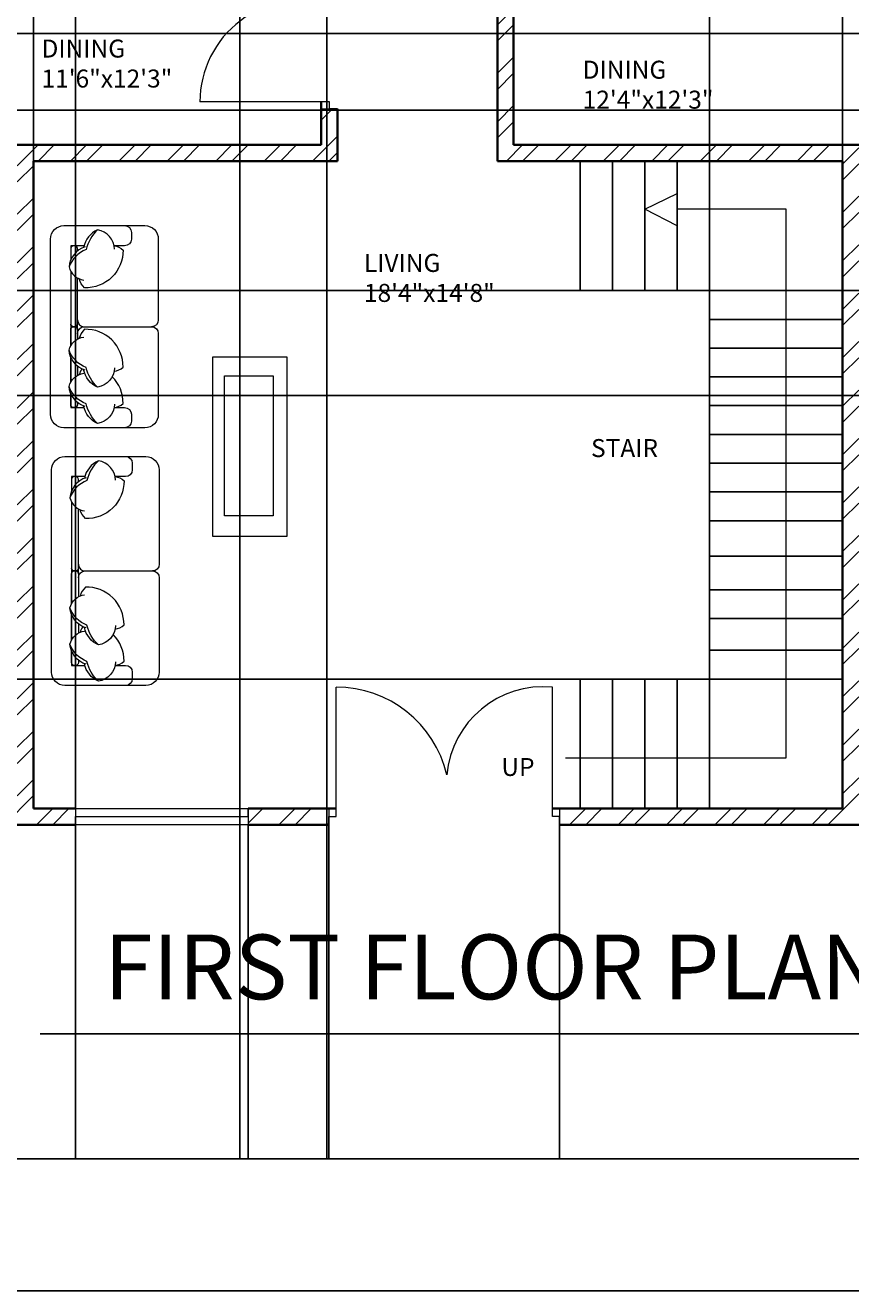
# Model space of a CAD drawing. Units: inches. Extents: x 1965 to 2673, y 1802 to 2669.
# Tile 4 of 16: x 2198 to 2427, y 1802 to 2154. Entities that reach past the tile are written whole.
import ezdxf

# ---------------------------------------------------------------- set-up
doc = ezdxf.new("R2010")
doc.units = ezdxf.units.IN
for name, color, linetype, lineweight in [('A-ANNO-DIMS', 2, 'Continuous', 18), ('A-ANNO-SYMB', 7, 'Continuous', 18), ('A-ANNO-TTLB', 7, 'Continuous', 25), ('A-AREA-IDEN', 7, 'Continuous', 18), ('A-DOOR', 11, 'Continuous', 18), ('A-FLOR-STRS', 131, 'Continuous', 25), ('A-FURN', 8, 'Continuous', 13), ('A-GLAZ', 181, 'Continuous', 18), ('A-WALL', 7, 'Continuous', 35), ('A-WALL-PATT', 252, 'Continuous', 13)]:
    doc.layers.add(name, color=color, linetype=linetype, lineweight=lineweight)
doc.styles.get("Standard").update_dxf_attribs({"font": 'arial.ttf'})
doc.dimstyles.get("Standard").update_dxf_attribs({"dimtxt": 0.18, "dimasz": 0.18, "dimexe": 0.18, "dimexo": 0.0625, "dimgap": 0.09, "dimtad": 0, "dimtih": 1, "dimtoh": 1, "dimdec": 4, "dimzin": 0, "dimdsep": 46, "dimtxsty": 'Standard', "dimcen": 0.09, "dimadec": 0, "dimazin": 0, "dimtfac": 1, "dimtdec": 4, "dimtofl": 0, "dimtmove": 0, "dimatfit": 3, "dimfxl": 1, "dimtolj": 1, "dimtzin": 0, "dimarcsym": 0})

# ---------------------------------------------------------------- blocks, each defined once
blk = doc.blocks.new('*D25')
at = {"layer": 'A-ANNO-DIMS', "color": 0, "lineweight": -2, "transparency": 16777216}
for p, q in [((2047.09, 1931.53), (2047.09, 1838.49)), ((2578.09, 1931.53), (2578.09, 1838.49)), ((2047.27, 1838.67), (2312.32, 1838.67)), ((2577.91, 1838.67), (2312.86, 1838.67))]:
    blk.add_line(p, q, dxfattribs=at)
at = {"layer": 'A-ANNO-DIMS', "color": 0, "transparency": 16777216}
for points in [[(2047.27, 1838.7), (2047.27, 1838.64), (2047.09, 1838.67)], [(2577.91, 1838.7), (2577.91, 1838.64), (2578.09, 1838.67)]]:
    blk.add_solid(points, dxfattribs=at)
at = {"layer": 'Defpoints', "color": 0, "transparency": 16777216}
for p in [(2047.09, 1931.59), (2578.09, 1931.59), (2578.09, 1838.67)]:
    blk.add_point(p, dxfattribs=at)
at = {"layer": 'A-ANNO-DIMS', "color": 0, "transparency": 16777216, "insert": (2312.59, 1838.67), "char_height": 0.18, "attachment_point": 5}
blk.add_mtext('\\A1;531', dxfattribs=at)
blk = doc.blocks.new('*D40')
at = {"layer": 'A-ANNO-DIMS', "color": 0, "lineweight": -2, "transparency": 16777216}
for p, q in [((2200.09, 1936.15), (2200.09, 2600.5)), ((2200.27, 2600.32), (2205.48, 2600.32)), ((2211.59, 2600.32), (2206.38, 2600.32)), ((2211.77, 1936.15), (2211.77, 2600.5))]:
    blk.add_line(p, q, dxfattribs=at)
at = {"layer": 'A-ANNO-DIMS', "color": 0, "transparency": 16777216}
for points in [[(2200.27, 2600.35), (2200.27, 2600.29), (2200.09, 2600.32)], [(2211.59, 2600.35), (2211.59, 2600.29), (2211.77, 2600.32)]]:
    blk.add_solid(points, dxfattribs=at)
at = {"layer": 'Defpoints', "color": 0, "transparency": 16777216}
for p in [(2211.77, 2600.32), (2200.09, 1936.09), (2211.77, 1936.09)]:
    blk.add_point(p, dxfattribs=at)
at = {"layer": 'A-ANNO-DIMS', "color": 0, "transparency": 16777216, "insert": (2205.93, 2600.32), "char_height": 0.18, "attachment_point": 5}
blk.add_mtext('\\A1;11.674', dxfattribs=at)
blk = doc.blocks.new('*D41')
at = {"layer": 'A-ANNO-DIMS', "color": 0, "lineweight": -2, "transparency": 16777216}
for p, q in [((2211.77, 1931.53), (2211.77, 1838.49)), ((2259.77, 1931.53), (2259.77, 1838.49)), ((2211.95, 1838.67), (2235.54, 1838.67)), ((2259.59, 1838.67), (2235.99, 1838.67))]:
    blk.add_line(p, q, dxfattribs=at)
at = {"layer": 'A-ANNO-DIMS', "color": 0, "transparency": 16777216}
for points in [[(2211.95, 1838.7), (2211.95, 1838.64), (2211.77, 1838.67)], [(2259.59, 1838.7), (2259.59, 1838.64), (2259.77, 1838.67)]]:
    blk.add_solid(points, dxfattribs=at)
at = {"layer": 'Defpoints', "color": 0, "transparency": 16777216}
for p in [(2211.77, 1931.59), (2259.77, 1931.59), (2259.77, 1838.67)]:
    blk.add_point(p, dxfattribs=at)
at = {"layer": 'A-ANNO-DIMS', "color": 0, "transparency": 16777216, "insert": (2235.77, 1838.67), "char_height": 0.18, "attachment_point": 5}
blk.add_mtext('\\A1;48', dxfattribs=at)
blk = doc.blocks.new('*D42')
at = {"layer": 'A-ANNO-DIMS', "color": 0, "lineweight": -2, "transparency": 16777216}
for p, q in [((2259.77, 1931.53), (2259.77, 1838.49)), ((2282.25, 1931.53), (2282.25, 1838.49)), ((2259.95, 1838.67), (2270.54, 1838.67)), ((2282.07, 1838.67), (2271.47, 1838.67))]:
    blk.add_line(p, q, dxfattribs=at)
at = {"layer": 'A-ANNO-DIMS', "color": 0, "transparency": 16777216}
for points in [[(2259.95, 1838.7), (2259.95, 1838.64), (2259.77, 1838.67)], [(2282.07, 1838.7), (2282.07, 1838.64), (2282.25, 1838.67)]]:
    blk.add_solid(points, dxfattribs=at)
at = {"layer": 'Defpoints', "color": 0, "transparency": 16777216}
for p in [(2259.77, 1931.59), (2282.25, 1931.59), (2282.25, 1838.67)]:
    blk.add_point(p, dxfattribs=at)
at = {"layer": 'A-ANNO-DIMS', "color": 0, "transparency": 16777216, "insert": (2271.01, 1838.67), "char_height": 0.18, "attachment_point": 5}
blk.add_mtext('\\A1;22.483', dxfattribs=at)
blk = doc.blocks.new('*D43')
at = {"layer": 'A-ANNO-DIMS', "color": 0, "lineweight": -2, "transparency": 16777216}
for p, q in [((2282.25, 1931.53), (2282.25, 1838.49)), ((2346.41, 1931.53), (2346.41, 1838.49)), ((2282.43, 1838.67), (2313.93, 1838.67)), ((2346.23, 1838.67), (2314.72, 1838.67))]:
    blk.add_line(p, q, dxfattribs=at)
at = {"layer": 'A-ANNO-DIMS', "color": 0, "transparency": 16777216}
for points in [[(2282.43, 1838.7), (2282.43, 1838.64), (2282.25, 1838.67)], [(2346.23, 1838.7), (2346.23, 1838.64), (2346.41, 1838.67)]]:
    blk.add_solid(points, dxfattribs=at)
at = {"layer": 'Defpoints', "color": 0, "transparency": 16777216}
for p in [(2282.25, 1931.59), (2346.41, 1931.59), (2346.41, 1838.67)]:
    blk.add_point(p, dxfattribs=at)
at = {"layer": 'A-ANNO-DIMS', "color": 0, "transparency": 16777216, "insert": (2314.33, 1838.67), "char_height": 0.18, "attachment_point": 5}
blk.add_mtext('\\A1;64.16', dxfattribs=at)
blk = doc.blocks.new('*D45')
at = {"layer": 'A-ANNO-DIMS', "color": 0, "lineweight": -2, "transparency": 16777216}
for p, q in [((2573.53, 2080.09), (2012.19, 2080.09)), ((2012.37, 2079.91), (2012.37, 2065.68)), ((2012.37, 2051.08), (2012.37, 2065.31)), ((2573.53, 2050.9), (2012.19, 2050.9))]:
    blk.add_line(p, q, dxfattribs=at)
at = {"layer": 'A-ANNO-DIMS', "color": 0, "transparency": 16777216}
for points in [[(2012.34, 2079.91), (2012.4, 2079.91), (2012.37, 2080.09)], [(2012.34, 2051.08), (2012.4, 2051.08), (2012.37, 2050.9)]]:
    blk.add_solid(points, dxfattribs=at)
at = {"layer": 'Defpoints', "color": 0, "transparency": 16777216}
for p in [(2012.37, 2080.09), (2573.59, 2080.09), (2573.59, 2050.9)]:
    blk.add_point(p, dxfattribs=at)
at = {"layer": 'A-ANNO-DIMS', "color": 0, "transparency": 16777216, "insert": (2012.37, 2065.49), "char_height": 0.18, "attachment_point": 5}
blk.add_mtext('\\A1;29.19', dxfattribs=at)
blk = doc.blocks.new('*D46')
at = {"layer": 'A-ANNO-DIMS', "color": 0, "lineweight": -2, "transparency": 16777216}
for p, q in [((2573.53, 2151.59), (2012.19, 2151.59)), ((2012.37, 2151.41), (2012.37, 2141.12)), ((2012.37, 2130.47), (2012.37, 2140.76)), ((2573.53, 2130.29), (2012.19, 2130.29))]:
    blk.add_line(p, q, dxfattribs=at)
at = {"layer": 'A-ANNO-DIMS', "color": 0, "transparency": 16777216}
for points in [[(2012.34, 2151.41), (2012.4, 2151.41), (2012.37, 2151.59)], [(2012.34, 2130.47), (2012.4, 2130.47), (2012.37, 2130.29)]]:
    blk.add_solid(points, dxfattribs=at)
at = {"layer": 'Defpoints', "color": 0, "transparency": 16777216}
for p in [(2012.37, 2151.59), (2573.59, 2151.59), (2573.59, 2130.29)]:
    blk.add_point(p, dxfattribs=at)
at = {"layer": 'A-ANNO-DIMS', "color": 0, "transparency": 16777216, "insert": (2012.37, 2140.94), "char_height": 0.18, "attachment_point": 5}
blk.add_mtext('\\A1;21.3', dxfattribs=at)
blk = doc.blocks.new('*D50')
at = {"layer": 'A-ANNO-DIMS', "color": 0, "lineweight": -2, "transparency": 16777216}
for p, q in [((2388.09, 2116.15), (2388.09, 2600.5)), ((2388.27, 2600.32), (2406.37, 2600.32)), ((2424.91, 2600.32), (2406.81, 2600.32)), ((2425.09, 2116.15), (2425.09, 2600.5))]:
    blk.add_line(p, q, dxfattribs=at)
at = {"layer": 'A-ANNO-DIMS', "color": 0, "transparency": 16777216}
for points in [[(2388.27, 2600.35), (2388.27, 2600.29), (2388.09, 2600.32)], [(2424.91, 2600.35), (2424.91, 2600.29), (2425.09, 2600.32)]]:
    blk.add_solid(points, dxfattribs=at)
at = {"layer": 'Defpoints', "color": 0, "transparency": 16777216}
for p in [(2425.09, 2600.32), (2388.09, 2116.09), (2425.09, 2116.09)]:
    blk.add_point(p, dxfattribs=at)
at = {"layer": 'A-ANNO-DIMS', "color": 0, "transparency": 16777216, "insert": (2406.59, 2600.32), "char_height": 0.18, "attachment_point": 5}
blk.add_mtext('\\A1;37', dxfattribs=at)
blk = doc.blocks.new('*D51')
at = {"layer": 'A-ANNO-DIMS', "color": 0, "lineweight": -2, "transparency": 16777216}
for p, q in [((2388.03, 2080.09), (2012.19, 2080.09)), ((2012.37, 2079.91), (2012.37, 2026.27)), ((2012.37, 1972.27), (2012.37, 2025.91)), ((2388.03, 1972.09), (2012.19, 1972.09))]:
    blk.add_line(p, q, dxfattribs=at)
at = {"layer": 'A-ANNO-DIMS', "color": 0, "transparency": 16777216}
for points in [[(2012.34, 2079.91), (2012.4, 2079.91), (2012.37, 2080.09)], [(2012.34, 1972.27), (2012.4, 1972.27), (2012.37, 1972.09)]]:
    blk.add_solid(points, dxfattribs=at)
at = {"layer": 'Defpoints', "color": 0, "transparency": 16777216}
for p in [(2012.37, 2080.09), (2388.09, 2080.09), (2388.09, 1972.09)]:
    blk.add_point(p, dxfattribs=at)
at = {"layer": 'A-ANNO-DIMS', "color": 0, "transparency": 16777216, "insert": (2012.37, 2026.09), "char_height": 0.18, "attachment_point": 5}
blk.add_mtext('\\A1;108', dxfattribs=at)
blk = doc.blocks.new('*D53')
at = {"layer": 'A-ANNO-DIMS', "color": 0, "lineweight": -2, "transparency": 16777216}
for p, q in [((2257.52, 2457.53), (2257.52, 1838.49)), ((2281.66, 2457.53), (2281.66, 1838.49)), ((2257.7, 1838.67), (2269.12, 1838.67)), ((2281.48, 1838.67), (2270.05, 1838.67))]:
    blk.add_line(p, q, dxfattribs=at)
at = {"layer": 'A-ANNO-DIMS', "color": 0, "transparency": 16777216}
for points in [[(2257.7, 1838.7), (2257.7, 1838.64), (2257.52, 1838.67)], [(2281.48, 1838.7), (2281.48, 1838.64), (2281.66, 1838.67)]]:
    blk.add_solid(points, dxfattribs=at)
at = {"layer": 'Defpoints', "color": 0, "transparency": 16777216}
for p in [(2257.52, 2457.59), (2281.66, 2457.59), (2281.66, 1838.67)]:
    blk.add_point(p, dxfattribs=at)
at = {"layer": 'A-ANNO-DIMS', "color": 0, "transparency": 16777216, "insert": (2269.59, 1838.67), "char_height": 0.18, "attachment_point": 5}
blk.add_mtext('\\A1;24.145', dxfattribs=at)

msp = doc.modelspace()

# ---------------------------------------------------------------- hatches: boundary and pattern name
at = {"layer": 'A-WALL-PATT'}
h = msp.add_hatch(dxfattribs=at)
h.set_pattern_fill('ANSI32', color=256)
h.paths.add_polyline_path([(2051.5927, 2561.0914), (2076.7559, 2561.0914), (2076.7559, 2563.3414), (2076.7559, 2565.5914), (2047.0927, 2565.5914), (2047.0927, 2518.3824), (2051.5927, 2518.3824)])
h.paths.add_polyline_path([(2051.5927, 2458.3824), (2049.3427, 2458.3824), (2047.0927, 2458.3824), (2047.0927, 2412.5914), (2248.0927, 2412.5914), (2248.0927, 2268.5914), (2252.5927, 2268.5914), (2252.5927, 2412.5914), (2252.5927, 2421.0404), (2250.3427, 2421.0404), (2248.0927, 2421.0404), (2248.0927, 2417.0914), (2051.5927, 2417.0914)])
h.paths.add_polyline_path([(2211.4933, 2268.5914), (2104.0927, 2268.5914), (2104.0927, 2272.4654), (2101.8427, 2272.4654), (2099.5927, 2272.4654), (2099.5927, 2268.5914), (2051.5927, 2268.5914), (2051.5927, 2264.0914), (2147.5927, 2264.0914), (2147.5927, 2259.8893), (2152.0927, 2259.8893), (2152.0927, 2264.0914), (2211.4933, 2264.0914), (2211.4933, 2266.3414)])
h.paths.add_polyline_path([(2104.0927, 2376.0914), (2099.5927, 2376.0914), (2047.0927, 2376.0914), (2047.0927, 2333.0682), (2051.5927, 2333.0682), (2051.5927, 2371.5914), (2099.5927, 2371.5914), (2099.5927, 2293.6123), (2104.0927, 2293.6123)], flags=17)
h.paths.add_polyline_path([(2051.5927, 2309.0682), (2047.0927, 2309.0682), (2047.0927, 2233.5821), (2051.5927, 2233.5821)])
h.paths.add_polyline_path([(2104.0927, 2412.5914), (2099.5927, 2412.5914), (2099.5927, 2376.0914), (2104.0927, 2376.0914)], flags=17)
h.paths.add_polyline_path([(2290.1254, 2268.5914), (2242.4924, 2268.5914), (2242.4924, 2264.0914), (2290.1254, 2264.0914), (2290.1254, 2266.3414)])
h.paths.add_polyline_path([(2284.653, 2264.0914), (2280.153, 2264.0914), (2280.153, 2161.6826), (2284.653, 2161.6826)])
h.paths.add_polyline_path([(2578.0927, 2329.4656), (2573.5927, 2329.4656), (2573.5927, 2268.5914), (2525.5927, 2268.5914), (2525.5927, 2271.9222), (2523.3427, 2271.9222), (2521.0927, 2271.9222), (2521.0927, 2268.5914), (2324.2835, 2268.5914), (2324.2835, 2264.0914), (2329.0927, 2264.0914), (2329.0927, 2259.4977), (2333.5927, 2259.4977), (2333.5927, 2264.0914), (2473.0927, 2264.0914), (2473.0927, 2259.9371), (2477.5927, 2259.9371), (2477.5927, 2264.0914), (2573.5927, 2264.0914), (2573.5927, 2235.5751), (2578.0927, 2235.5751)])
h.paths.add_polyline_path([(2377.0927, 2412.5914), (2578.0927, 2412.5914), (2578.0927, 2444.2286), (2575.8427, 2444.2286), (2573.5927, 2444.2286), (2573.5927, 2417.0914), (2429.5927, 2417.0914), (2377.0927, 2417.0914), (2377.0927, 2421.7443), (2372.5927, 2421.7443), (2372.5927, 2268.5914), (2377.0927, 2268.5914)])
h.paths.add_polyline_path([(2525.5927, 2371.5914), (2573.5927, 2371.5914), (2573.5927, 2353.4656), (2578.0927, 2353.4656), (2578.0927, 2376.0914), (2525.5927, 2376.0914), (2521.0927, 2376.0914), (2521.0927, 2290.6472), (2525.5927, 2290.6472)], flags=17)
h.paths.add_polyline_path([(2477.5927, 2236.4106), (2475.3427, 2236.4106), (2473.0927, 2236.4106), (2473.0927, 2084.5914), (2465.3309, 2084.5914), (2465.3309, 2080.0914), (2481.6764, 2080.0914), (2481.6764, 2082.3414), (2481.6764, 2084.5914), (2477.5927, 2084.5914), (2477.5927, 2151.5914), (2573.5927, 2151.5914), (2573.5927, 2130.2907), (2578.0927, 2130.2907), (2578.0927, 2199.5751), (2575.8427, 2199.5751), (2573.5927, 2199.5751), (2573.5927, 2156.0914), (2477.5927, 2156.0914)])
h.paths.add_polyline_path([(2573.5927, 2084.5914), (2505.5513, 2084.5914), (2505.5513, 2080.0914), (2573.5927, 2080.0914)], flags=17)
h.paths.add_polyline_path([(2578.0927, 2106.2907), (2575.8427, 2106.2907), (2573.5927, 2106.2907), (2573.5927, 2050.8986), (2578.0927, 2050.8986)])
h.paths.add_polyline_path([(2578.0927, 1990.8986), (2575.8427, 1990.8986), (2573.5927, 1990.8986), (2573.5927, 1936.0914), (2522.132, 1936.0914), (2522.132, 1931.5914), (2578.0927, 1931.5914)])
h.paths.add_polyline_path([(2462.132, 1936.0914), (2429.5927, 1936.0914), (2429.5927, 2080.0914), (2432.623, 2080.0914), (2432.623, 2082.3414), (2432.623, 2084.5914), (2429.5927, 2084.5914), (2429.5927, 2120.5914), (2333.5927, 2120.5914), (2333.5927, 2229.3125), (2331.3427, 2229.3125), (2329.0927, 2229.3125), (2329.0927, 2116.0914), (2425.0927, 2116.0914), (2425.0927, 1936.0914), (2346.4058, 1936.0914), (2346.4058, 1931.5914), (2462.132, 1931.5914), (2462.132, 1933.8414)])
h.paths.add_polyline_path([(2211.767, 1933.8414), (2211.767, 1936.0914), (2200.0927, 1936.0914), (2200.0927, 2080.0914), (2200.0927, 2116.0914), (2284.653, 2116.0914), (2284.653, 2130.591), (2282.403, 2130.591), (2280.153, 2130.591), (2280.153, 2120.5914), (2200.0927, 2120.5914), (2195.5927, 2120.5914), (2195.5927, 2080.0914), (2195.5927, 1936.0914), (2139.0533, 1936.0914), (2139.0533, 1931.5914), (2211.767, 1931.5914)])
h.paths.add_polyline_path([(2282.2502, 1933.8414), (2282.2502, 1936.0914), (2259.767, 1936.0914), (2259.767, 1931.5914), (2282.2502, 1931.5914)], flags=17)
h.paths.add_polyline_path([(2051.5927, 1987.096), (2049.3427, 1987.096), (2047.0927, 1987.096), (2047.0927, 1931.5914), (2079.0533, 1931.5914), (2079.0533, 1933.8414), (2079.0533, 1936.0914), (2051.5927, 1936.0914)])
h.paths.add_polyline_path([(2051.5927, 2197.5821), (2049.3427, 2197.5821), (2047.0927, 2197.5821), (2047.0927, 2141.952), (2051.5927, 2141.952), (2051.5927, 2151.5914), (2147.5927, 2151.5914), (2147.5927, 2084.5914), (2144.3652, 2084.5914), (2144.3652, 2080.0914), (2155.9662, 2080.0914), (2155.9662, 2082.3414), (2155.9662, 2084.5914), (2152.0927, 2084.5914), (2152.0927, 2239.4921), (2149.8427, 2239.4921), (2147.5927, 2239.4921), (2147.5927, 2156.0914), (2051.5927, 2156.0914)])
h.paths.add_polyline_path([(2051.5927, 2080.0914), (2123.8575, 2080.0914), (2123.8575, 2082.3414), (2123.8575, 2084.5914), (2051.5927, 2084.5914), (2051.5927, 2117.952), (2047.0927, 2117.952), (2047.0927, 2047.096), (2051.5927, 2047.096)])
h = msp.add_hatch(dxfattribs=at)
h.set_pattern_fill('ANSI32', color=256)
h.paths.add_polyline_path([(2210.2316, 2563.3414), (2210.2316, 2565.5914), (2136.7559, 2565.5914), (2136.7559, 2561.0914), (2195.5927, 2561.0914), (2195.5927, 2485.8604), (2200.0927, 2485.8604), (2200.0927, 2561.0914), (2210.2316, 2561.0914)])
h.paths.add_polyline_path([(2285.9734, 2565.5914), (2234.2316, 2565.5914), (2234.2316, 2561.0914), (2248.0927, 2561.0914), (2248.0927, 2462.0914), (2200.0927, 2462.0914), (2200.0927, 2465.2357), (2197.8427, 2465.2357), (2195.5927, 2465.2357), (2195.5927, 2457.5914), (2248.0927, 2457.5914), (2248.0927, 2452.628), (2252.5927, 2452.628), (2252.5927, 2457.5914), (2257.5156, 2457.5914), (2257.5156, 2459.8414), (2257.5156, 2462.0914), (2252.5927, 2462.0914), (2252.5927, 2561.0914), (2285.9734, 2561.0914)])
h.paths.add_polyline_path([(2213.1374, 1872.8885), (2461.061, 1872.8885), (2461.061, 1909.9813), (2213.1374, 1909.9813)], flags=9)
h.paths.add_polyline_path([(2328.4056, 1942.3944), (2340.6089, 1942.3944), (2340.6089, 1952.6979), (2328.4056, 1952.6979)], flags=9)
h.paths.add_polyline_path([(2353.5759, 2030.9808), (2376.6455, 2030.9808), (2376.6455, 2041.2844), (2353.5759, 2041.2844)], flags=9)
h.paths.add_polyline_path([(2289.989, 2074.1041), (2326.916, 2074.1041), (2326.916, 2092.7615), (2289.989, 2092.7615)], flags=9)
h.paths.add_polyline_path([(2497.9, 2052.8638), (2548.3741, 2052.8638), (2548.3741, 2071.5212), (2497.9, 2071.5212)], flags=9)
h.paths.add_polyline_path([(2486.59, 2116.4883), (2515.7475, 2116.4883), (2515.7475, 2135.1456), (2486.59, 2135.1456)], flags=9)
h.paths.add_polyline_path([(2497.3007, 2181.2877), (2530.459, 2181.2877), (2530.459, 2199.945), (2497.3007, 2199.945)], flags=9)
h.paths.add_polyline_path([(2288.237, 2190.3228), (2324.1238, 2190.3228), (2324.1238, 2208.9802), (2288.237, 2208.9802)], flags=9)
h.paths.add_polyline_path([(2350.806, 2127.8307), (2387.733, 2127.8307), (2387.733, 2146.488), (2350.806, 2146.488)], flags=9)
h.paths.add_polyline_path([(2530.3237, 2315.2679), (2559.5563, 2315.2679), (2559.5563, 2333.9252), (2530.3237, 2333.9252)], flags=9)
h.paths.add_polyline_path([(2418.419, 2383.4707), (2468.2894, 2383.4707), (2468.2894, 2402.1281), (2418.419, 2402.1281)], flags=9)
h.paths.add_polyline_path([(2327.4503, 2399.0281), (2364.3773, 2399.0281), (2364.3773, 2417.6854), (2327.4503, 2417.6854)], flags=9)
h.paths.add_polyline_path([(2147.9722, 2271.4601), (2197.8426, 2271.4601), (2197.8426, 2290.1174), (2147.9722, 2290.1174)], flags=9)
h.paths.add_polyline_path([(2474.3875, 2421.594), (2524.8616, 2421.594), (2524.8616, 2440.2514), (2474.3875, 2440.2514)], flags=9)
h.paths.add_polyline_path([(2063.9863, 2052.9059), (2114.4604, 2052.9059), (2114.4604, 2071.5632), (2063.9863, 2071.5632)], flags=9)
h.paths.add_polyline_path([(2200.3335, 2133.7067), (2237.2605, 2133.7067), (2237.2605, 2152.364), (2200.3335, 2152.364)], flags=9)
h.paths.add_polyline_path([(2080.5973, 2184.636), (2113.8681, 2184.636), (2113.8681, 2203.2933), (2080.5973, 2203.2933)], flags=9)
h.paths.add_polyline_path([(2102.4918, 2116.4497), (2131.6494, 2116.4497), (2131.6494, 2135.107), (2102.4918, 2135.107)], flags=9)
h.paths.add_polyline_path([(2056.2753, 2308.5576), (2085.5079, 2308.5576), (2085.5079, 2327.2149), (2056.2753, 2327.2149)], flags=9)
h.paths.add_polyline_path([(2385.619, 2500.9729), (2414.8516, 2500.9729), (2414.8516, 2519.6303), (2385.619, 2519.6303)], flags=9)
h.paths.add_polyline_path([(2286.6643, 2508.6826), (2320.0715, 2508.6826), (2320.0715, 2527.34), (2286.6643, 2527.34)], flags=9)
h.paths.add_polyline_path([(2206.5604, 2500.7243), (2235.793, 2500.7243), (2235.793, 2519.3817), (2206.5604, 2519.3817)], flags=25)
h.paths.add_polyline_path([(2062.6644, 2424.4027), (2112.5348, 2424.4027), (2112.5348, 2443.0601), (2062.6644, 2443.0601)], flags=9)
h = msp.add_hatch(dxfattribs=at)
h.set_pattern_fill('ANSI32', color=256)
h.paths.add_polyline_path([(2429.5927, 2468.6101), (2427.3427, 2468.6101), (2425.0927, 2468.6101), (2425.0927, 2462.0914), (2377.0927, 2462.0914), (2377.0927, 2561.0914), (2390.4173, 2561.0914), (2390.4173, 2565.5914), (2321.9734, 2565.5914), (2321.9734, 2561.0914), (2372.5927, 2561.0914), (2372.5927, 2462.0914), (2281.6605, 2462.0914), (2281.6605, 2457.5914), (2372.5927, 2457.5914), (2372.5927, 2451.3316), (2377.0927, 2451.3316), (2377.0927, 2457.5914), (2429.5927, 2457.5914)])
h.paths.add_polyline_path([(2480.8929, 2565.5914), (2414.4173, 2565.5914), (2414.4173, 2561.0914), (2425.0927, 2561.0914), (2425.0927, 2489.9153), (2429.5927, 2489.9153), (2429.5927, 2561.0914), (2480.8929, 2561.0914), (2480.8929, 2563.3414)])
h.paths.add_polyline_path([(2213.1374, 1872.8885), (2461.061, 1872.8885), (2461.061, 1909.9813), (2213.1374, 1909.9813)], flags=9)
h.paths.add_polyline_path([(2328.4056, 1942.3944), (2340.6089, 1942.3944), (2340.6089, 1952.6979), (2328.4056, 1952.6979)], flags=9)
h.paths.add_polyline_path([(2353.5759, 2030.9808), (2376.6455, 2030.9808), (2376.6455, 2041.2844), (2353.5759, 2041.2844)], flags=9)
h.paths.add_polyline_path([(2289.989, 2074.1041), (2326.916, 2074.1041), (2326.916, 2092.7615), (2289.989, 2092.7615)], flags=9)
h.paths.add_polyline_path([(2497.9, 2052.8638), (2548.3741, 2052.8638), (2548.3741, 2071.5212), (2497.9, 2071.5212)], flags=9)
h.paths.add_polyline_path([(2486.59, 2116.4883), (2515.7475, 2116.4883), (2515.7475, 2135.1456), (2486.59, 2135.1456)], flags=9)
h.paths.add_polyline_path([(2497.3007, 2181.2877), (2530.459, 2181.2877), (2530.459, 2199.945), (2497.3007, 2199.945)], flags=9)
h.paths.add_polyline_path([(2288.237, 2190.3228), (2324.1238, 2190.3228), (2324.1238, 2208.9802), (2288.237, 2208.9802)], flags=9)
h.paths.add_polyline_path([(2350.806, 2127.8307), (2387.733, 2127.8307), (2387.733, 2146.488), (2350.806, 2146.488)], flags=9)
h.paths.add_polyline_path([(2530.3237, 2315.2679), (2559.5563, 2315.2679), (2559.5563, 2333.9252), (2530.3237, 2333.9252)], flags=9)
h.paths.add_polyline_path([(2418.419, 2383.4707), (2468.2894, 2383.4707), (2468.2894, 2402.1281), (2418.419, 2402.1281)], flags=9)
h.paths.add_polyline_path([(2327.4503, 2399.0281), (2364.3773, 2399.0281), (2364.3773, 2417.6854), (2327.4503, 2417.6854)], flags=9)
h.paths.add_polyline_path([(2147.9722, 2271.4601), (2197.8426, 2271.4601), (2197.8426, 2290.1174), (2147.9722, 2290.1174)], flags=9)
h.paths.add_polyline_path([(2474.3875, 2421.594), (2524.8616, 2421.594), (2524.8616, 2440.2514), (2474.3875, 2440.2514)], flags=9)
h.paths.add_polyline_path([(2063.9863, 2052.9059), (2114.4604, 2052.9059), (2114.4604, 2071.5632), (2063.9863, 2071.5632)], flags=9)
h.paths.add_polyline_path([(2200.3335, 2133.7067), (2237.2605, 2133.7067), (2237.2605, 2152.364), (2200.3335, 2152.364)], flags=9)
h.paths.add_polyline_path([(2080.5973, 2184.636), (2113.8681, 2184.636), (2113.8681, 2203.2933), (2080.5973, 2203.2933)], flags=9)
h.paths.add_polyline_path([(2102.4918, 2116.4497), (2131.6494, 2116.4497), (2131.6494, 2135.107), (2102.4918, 2135.107)], flags=9)
h.paths.add_polyline_path([(2056.2753, 2308.5576), (2085.5079, 2308.5576), (2085.5079, 2327.2149), (2056.2753, 2327.2149)], flags=9)
h.paths.add_polyline_path([(2385.619, 2500.9729), (2414.8516, 2500.9729), (2414.8516, 2519.6303), (2385.619, 2519.6303)], flags=25)
h.paths.add_polyline_path([(2286.6643, 2508.6826), (2320.0715, 2508.6826), (2320.0715, 2527.34), (2286.6643, 2527.34)], flags=25)
h.paths.add_polyline_path([(2206.5604, 2500.7243), (2235.793, 2500.7243), (2235.793, 2519.3817), (2206.5604, 2519.3817)], flags=9)
h.paths.add_polyline_path([(2062.6644, 2424.4027), (2112.5348, 2424.4027), (2112.5348, 2443.0601), (2062.6644, 2443.0601)], flags=9)

# ---------------------------------------------------------------- linework, layer by layer
at = {"layer": 'A-ANNO-SYMB'}
for p, q in [((2370.0925, 2102.6772), (2379.0925, 2107.0674)), ((2379.0925, 2107.0674), (2379.0925, 2098.0914)), ((2379.0925, 2098.0914), (2370.0925, 2102.6772)), ((2409.396, 2102.6772), (2379.0925, 2102.6772)), ((2409.396, 1950.1498), (2409.396, 2102.6772)), ((2348.0205, 1950.1498), (2409.396, 1950.1498))]:
    msp.add_line(p, q, dxfattribs=at)
at = {"layer": 'A-ANNO-TTLB'}
msp.add_line((2201.9386, 1873.3965), (2476.233, 1873.3965), dxfattribs=at)
msp.add_lwpolyline([(1964.5703, 2669.282), (2673.2605, 2669.282), (2673.2605, 1802.0221), (1964.5703, 1802.0221)], close=True, dxfattribs=at)
at = {"layer": 'A-DOOR'}
for p, q in [((2282.403, 2132.591), (2246.403, 2132.591)), ((2282.403, 2130.591), (2282.403, 2132.591)), ((2280.153, 2130.591), (2284.653, 2130.591)), ((2284.653, 2130.591), (2282.403, 2130.591)), ((2284.2502, 1933.8414), (2284.2502, 1969.8414)), ((2344.4058, 1933.8414), (2344.4058, 1969.8414)), ((2282.2502, 1936.0914), (2282.2502, 1931.5914)), ((2346.4058, 1936.0914), (2346.4058, 1931.5914)), ((2282.2502, 1931.5914), (2282.2502, 1933.8414)), ((2282.2502, 1933.8414), (2284.2502, 1933.8414)), ((2346.4058, 1933.8414), (2344.4058, 1933.8414)), ((2346.4058, 1931.5914), (2346.4058, 1933.8414))]:
    msp.add_line(p, q, dxfattribs=at)
for centre, radius, start, end in [((2274.5969, 2132.591), 28.1938, 73.926247, 180), ((2284.2502, 1938.2178), 31.6235, 13.210494, 90), ((2341.937, 1942.9377), 27.0167, 84.757023, 174.675446)]:
    msp.add_arc(centre, radius, start, end, dxfattribs=at)
at = {"layer": 'A-FLOR-STRS'}
for p, q in [((2352.0925, 2080.0914), (2352.0925, 2116.0914)), ((2361.0925, 2080.0914), (2361.0925, 2116.0914)), ((2370.0925, 2080.0914), (2370.0925, 2116.0914)), ((2379.0925, 2080.0914), (2379.0925, 2116.0914)), ((2388.0925, 1972.0914), (2388.0925, 2116.0914)), ((2388.0925, 2116.0914), (2388.0925, 2080.0914)), ((2388.0925, 2080.0914), (2388.0925, 2116.0914)), ((2388.0925, 2080.0914), (2352.0925, 2080.0914)), ((2388.0925, 2080.0914), (2425.0927, 2080.0914)), ((2388.0925, 2072.0914), (2425.0927, 2072.0914)), ((2388.0925, 2064.0914), (2425.0927, 2064.0914)), ((2388.0925, 2056.0914), (2425.0927, 2056.0914)), ((2388.0925, 2048.0914), (2425.0927, 2048.0914)), ((2388.0925, 2040.0914), (2425.0927, 2040.0914)), ((2388.0925, 2032.0914), (2425.0927, 2032.0914)), ((2388.0925, 2024.0914), (2425.0927, 2024.0914)), ((2388.0925, 2016.0914), (2425.0927, 2016.0914)), ((2388.0925, 2006.2051), (2425.0927, 2006.2051)), ((2388.0925, 1996.8719), (2425.0927, 1996.8719)), ((2388.0925, 1988.8719), (2425.0927, 1988.8719)), ((2388.0925, 1980.1388), (2425.0927, 1980.1388)), ((2352.0925, 1936.0914), (2352.0925, 1972.0914)), ((2352.0925, 1972.0914), (2425.0927, 1972.0914)), ((2361.0925, 1936.0914), (2361.0925, 1972.0914)), ((2370.0925, 1936.0914), (2370.0925, 1972.0914)), ((2379.0925, 1936.0914), (2379.0925, 1972.0914)), ((2388.0925, 1936.0914), (2388.0925, 1972.0914))]:
    msp.add_line(p, q, dxfattribs=at)
at = {"layer": 'A-FURN', "ltscale": 0.03}
for points in [[(2234.8301, 2071.9136, -0.41421356), (2232.9566, 2070.04, -0.41421356), (2234.8301, 2068.1664), (2234.8301, 2045.6834, -0.41421356), (2231.083, 2041.9363), (2208.6, 2041.9363, -0.41421356), (2204.8528, 2045.6834), (2204.8528, 2094.3966, -0.41421356), (2208.6, 2098.1437), (2231.083, 2098.1437, -0.41421356), (2234.8301, 2094.3966), (2234.8301, 2071.9136, -0.41421356), (2232.9566, 2070.04, -0.41421356), (2234.8301, 2068.1664)], [(2235.0818, 2003.9953, -0.41421356), (2233.2083, 2002.1217, -0.41421356), (2235.0818, 2000.2481), (2235.0818, 1974.018, -0.41421356), (2231.3347, 1970.2708), (2208.8517, 1970.2708, -0.41421356), (2205.1045, 1974.018), (2205.1045, 2030.2254, -0.41421356), (2208.8517, 2033.9726), (2231.3347, 2033.9726, -0.41421356), (2235.0818, 2030.2254), (2235.0818, 2003.9953, -0.41421356), (2233.2083, 2002.1217, -0.41421356), (2235.0818, 2000.2481)]]:
    msp.add_lwpolyline(points, format="xyb", dxfattribs=at)
at = {"layer": 'A-FURN'}
for points in [[(2217.9502, 2096.9513, 0.14772988), (2214.7302, 2091.4754, 0.21334276), (2210.0077, 2086.6437, 0.17866181)], [(2222.6728, 2091.5827, 0.35677236), (2217.9502, 2096.9513, 0.24954205), (2214.0584, 2092.0869, -9.61688035)], [(2225.4622, 2098.1437, -0.41421356), (2227.3358, 2096.2701), (2227.3358, 2094.3966, -0.41421356), (2225.4622, 2092.523), (2222.5594, 2092.523)], [(2214.4736, 2092.2319, 0.30666349), (2210.0077, 2086.6437, 0.30632997), (2214.0862, 2082.993, -0.87284716)], [(2212.3472, 2091.0932), (2212.3472, 2091.7735, 0.41421356), (2211.5977, 2092.523), (2211.223, 2092.523, 0.41421356), (2210.4736, 2091.7735)], [(2210.4736, 2091.7735), (2210.4736, 2088.5815, 0.41421356)], [(2222.5585, 2092.5271, -0.16554063), (2225.034, 2091.368, -0.42598917), (2214.3009, 2080.8456, -0.12152332), (2212.8215, 2083.3434, 7.11546429)], [(2210.4736, 2085.4645), (2210.4736, 2070.7894, 0.41421356), (2211.223, 2070.04), (2211.5977, 2070.04, 0.41421356), (2212.3472, 2070.7894), (2212.3472, 2083.5779, 0.41421356)], [(2210.4736, 2064.7084), (2210.4736, 2069.2906, -0.41421356), (2211.223, 2070.04), (2211.5977, 2070.04, -0.41421356), (2212.3472, 2069.2906), (2212.3472, 2066.595, -0.41421356)], [(2212.3472, 2071.9136, 0.41421356), (2214.2207, 2070.04)], [(2212.3472, 2071.9136, 0.41421356), (2214.2207, 2070.04), (2232.9566, 2070.04, 0.41421356)], [(2212.3472, 2068.1664, -0.41421356), (2214.2207, 2070.04)], [(2212.3472, 2068.1664, -0.41421356), (2214.2207, 2070.04), (2232.9566, 2070.04, -0.41421356)], [(2222.5585, 2057.6459, 0.16554063), (2225.034, 2058.8049, 0.42598917), (2214.3009, 2069.3273, 0.12152332), (2212.8215, 2066.8295, -7.11546429)], [(2214.4736, 2057.941, -0.30666349), (2210.0077, 2063.5293, -0.30632997), (2214.0862, 2067.1799, 0.87284716)], [(2217.9502, 2053.2216, -0.14772988), (2214.7302, 2058.6975, -0.21334276), (2210.0077, 2063.5293, -0.17866181)], [(2210.4736, 2054.6155), (2210.4736, 2061.5914, -0.41421356)], [(2212.3472, 2059.0797), (2212.3472, 2056.5021, -0.41421356)], [(2213.554, 2058.3074, 0.07186538), (2212.8215, 2056.7366, -7.11546429)], [(2222.6728, 2058.5902, -0.35677236), (2217.9502, 2053.2216, -0.24954205), (2214.0584, 2058.086, 9.61688035)], [(2214.4736, 2047.8481, -0.30666349), (2210.0077, 2053.4363, -0.30632997), (2214.0862, 2057.087, 0.87284716)], [(2222.5585, 2047.5529, 0.16554063), (2225.034, 2048.712, 0.20023115), (2222.0191, 2056.1494, 0.12152332)], [(2217.9502, 2043.1287, -0.14772988), (2214.7302, 2048.6046, -0.21334276), (2210.0077, 2053.4363, -0.17866181)], [(2210.4736, 2048.3064), (2210.4736, 2051.4985, -0.41421356)], [(2210.4736, 2051.4985), (2210.4736, 2047.557), (2214.1556, 2047.557, -0.41421356)], [(2212.3472, 2048.9868), (2212.3472, 2048.3064, -0.41421356), (2211.5977, 2047.557), (2211.223, 2047.557, -0.41421356), (2210.4736, 2048.3064)], [(2222.6728, 2048.4973, -0.35677236), (2217.9502, 2043.1287, -0.24954205), (2214.0584, 2047.9931, 9.61688035)], [(2222.5594, 2047.557), (2225.4622, 2047.557, -0.41421356), (2227.3358, 2045.6834), (2227.3358, 2043.8099, -0.41421356), (2225.4622, 2041.9363)], [(2225.7139, 2033.9726, -0.41421356), (2227.5875, 2032.099), (2227.5875, 2030.2254, -0.41421356), (2225.7139, 2028.3518), (2222.8111, 2028.3518)], [(2218.2019, 2032.7802, 0.14772988), (2214.9819, 2027.3042, 0.21334276), (2210.2594, 2022.4725, 0.17866181)], [(2222.9245, 2027.4116, 0.35677236), (2218.2019, 2032.7802, 0.24954205), (2214.3101, 2027.9158, -9.61688035)], [(2214.7253, 2028.0607, 0.30666349), (2210.2594, 2022.4725, 0.30632997), (2214.338, 2018.8219, -0.87284716)], [(2212.5989, 2026.9221), (2212.5989, 2027.6024, 0.41421356), (2211.8494, 2028.3518), (2211.4747, 2028.3518, 0.41421356), (2210.7253, 2027.6024)], [(2210.7253, 2027.6024), (2210.7253, 2024.4103, 0.41421356)], [(2222.8102, 2028.3559, -0.16554063), (2225.2857, 2027.1969, -0.42598917), (2214.5526, 2016.6745, -0.12152332), (2213.0732, 2019.1723, 7.11546429)], [(2210.7253, 2021.2934), (2210.7253, 2002.8711, 0.41421356), (2211.4747, 2002.1217), (2211.8494, 2002.1217, 0.41421356), (2212.5989, 2002.8711), (2212.5989, 2019.4068, 0.41421356)], [(2210.7253, 1993.0429), (2210.7253, 2001.3723, -0.41421356), (2211.4747, 2002.1217), (2211.8494, 2002.1217, -0.41421356), (2212.5989, 2001.3723), (2212.5989, 1994.9295, -0.41421356)], [(2212.5989, 2003.9953, 0.41421356), (2214.4724, 2002.1217)], [(2212.5989, 2003.9953, 0.41421356), (2214.4724, 2002.1217), (2233.2083, 2002.1217, 0.41421356)], [(2212.5989, 2000.2481, -0.41421356), (2214.4724, 2002.1217)], [(2212.5989, 2000.2481, -0.41421356), (2214.4724, 2002.1217), (2233.2083, 2002.1217, -0.41421356)], [(2214.7253, 1986.2756, -0.30666349), (2210.2594, 1991.8638, -0.30632997), (2214.338, 1995.5144, 0.87284716)], [(2222.8102, 1985.9804, 0.16554063), (2225.2857, 1987.1394, 0.42598917), (2214.5526, 1997.6618, 0.12152332), (2213.0732, 1995.164, -7.11546429)], [(2218.2019, 1981.5561, -0.14772988), (2214.9819, 1987.0321, -0.21334276), (2210.2594, 1991.8638, -0.17866181)], [(2210.7253, 1982.95), (2210.7253, 1989.926, -0.41421356)], [(2214.7253, 1976.1826, -0.30666349), (2210.2594, 1981.7709, -0.30632997), (2214.338, 1985.4215, 0.87284716)], [(2212.5989, 1987.4142), (2212.5989, 1984.8366, -0.41421356)], [(2213.8057, 1986.6419, 0.07186538), (2213.0732, 1985.0711, -7.11546429)], [(2222.9245, 1986.9247, -0.35677236), (2218.2019, 1981.5561, -0.24954205), (2214.3101, 1986.4205, 9.61688035)], [(2222.8102, 1975.8875, 0.16554063), (2225.2857, 1977.0465, 0.20023115), (2222.2708, 1984.484, 0.12152332)], [(2218.2019, 1971.4632, -0.14772988), (2214.9819, 1976.9392, -0.21334276), (2210.2594, 1981.7709, -0.17866181)], [(2210.7253, 1979.833), (2210.7253, 1975.8915), (2214.4073, 1975.8915, -0.41421356)], [(2210.7253, 1976.641), (2210.7253, 1979.833, -0.41421356)], [(2212.5989, 1977.3213), (2212.5989, 1976.641, -0.41421356), (2211.8494, 1975.8915), (2211.4747, 1975.8915, -0.41421356), (2210.7253, 1976.641)], [(2222.9245, 1976.8318, -0.35677236), (2218.2019, 1971.4632, -0.24954205), (2214.3101, 1976.3276, 9.61688035)], [(2222.8111, 1975.8915), (2225.7139, 1975.8915, -0.41421356), (2227.5875, 1974.018), (2227.5875, 1972.1444, -0.41421356), (2225.7139, 1970.2708)]]:
    msp.add_lwpolyline(points, format="xyb", dxfattribs=at)
for points in [[(2214.1556, 2092.523), (2210.4736, 2092.523), (2210.4736, 2088.5815)], [(2210.4736, 2085.4645), (2210.4736, 2064.7084)], [(2210.4736, 2061.5914), (2210.4736, 2054.6155)], [(2214.4073, 2028.3518), (2210.7253, 2028.3518), (2210.7253, 2024.4103)], [(2210.7253, 2021.2934), (2210.7253, 1993.0429)], [(2210.7253, 1989.926), (2210.7253, 1982.95)]]:
    msp.add_lwpolyline(points, dxfattribs=at)
for points in [[(2210.4736, 2070.7894), (2210.4736, 2069.2906, -0.41421356), (2211.223, 2070.04), (2211.5977, 2070.04, -0.41421356), (2212.3472, 2069.2906), (2212.3472, 2070.7894, -0.41421356), (2211.5977, 2070.04), (2211.223, 2070.04, -0.41421356)], [(2210.7253, 2002.8711), (2210.7253, 2001.3723, -0.41421356), (2211.4747, 2002.1217), (2211.8494, 2002.1217, -0.41421356), (2212.5989, 2001.3723), (2212.5989, 2002.8711, -0.41421356), (2211.8494, 2002.1217), (2211.4747, 2002.1217, -0.41421356)]]:
    msp.add_lwpolyline(points, format="xyb", close=True, dxfattribs=at)
for points in [[(2249.9973, 2061.6385), (2270.5146, 2061.6385), (2270.5146, 2011.7208), (2249.9973, 2011.7208)], [(2253.2669, 2056.3933), (2266.7834, 2056.3933), (2266.7834, 2017.4548), (2253.2669, 2017.4548)]]:
    msp.add_lwpolyline(points, close=True, dxfattribs=at)
at = {"layer": 'A-GLAZ'}
for p, q in [((2211.767, 1936.0914), (2211.767, 1931.5914)), ((2211.767, 1936.0914), (2259.767, 1936.0914)), ((2259.767, 1933.8414), (2259.767, 1936.0914)), ((2259.767, 1936.0914), (2259.767, 1931.5914)), ((2211.767, 1931.5914), (2211.767, 1933.8414)), ((2211.767, 1933.8414), (2259.767, 1933.8414)), ((2259.767, 1931.5914), (2211.767, 1931.5914))]:
    msp.add_line(p, q, dxfattribs=at)
at = {"layer": 'A-WALL'}
for p, q in [((2333.5927, 2230.6883), (2333.5927, 2120.5914)), ((2329.0927, 2229.3125), (2329.0927, 2116.0914)), ((2280.153, 2132.591), (2280.153, 2120.5914)), ((2284.653, 2130.591), (2284.653, 2116.0914)), ((2200.0927, 2120.5914), (2195.5927, 2120.5914)), ((2280.153, 2120.5914), (2200.0927, 2120.5914)), ((2329.0927, 2120.5914), (2329.0927, 2116.0914)), ((2429.5927, 2120.5914), (2333.5927, 2120.5914)), ((2200.0927, 2080.0914), (2200.0927, 2116.0914)), ((2200.0927, 2116.0914), (2284.653, 2116.0914)), ((2329.0927, 2116.0914), (2425.0927, 2116.0914)), ((2425.0927, 2116.0914), (2425.0927, 1936.0914)), ((2200.0927, 2080.0914), (2200.0927, 1936.0914)), ((2200.0927, 1936.0914), (2211.767, 1936.0914)), ((2259.767, 1936.0914), (2284.2502, 1936.0914)), ((2344.4058, 1936.0914), (2425.0927, 1936.0914)), ((2139.0533, 1931.5914), (2211.767, 1931.5914)), ((2259.767, 1931.5914), (2282.2502, 1931.5914)), ((2346.4058, 1931.5914), (2462.132, 1931.5914))]:
    msp.add_line(p, q, dxfattribs=at)

# ---------------------------------------------------------------- texts
at = {"layer": 'A-ANNO-SYMB', "insert": (2330.2047, 1950.1246), "char_height": 5, "attachment_point": 1}
msp.add_mtext_dynamic_manual_height_columns('UP', width=20.162846, gutter_width=12.5, heights=[0], dxfattribs=at)
at = {"layer": 'A-ANNO-TTLB', "insert": (2219.7001, 1901.0365), "char_height": 18, "attachment_point": 1}
msp.add_mtext_dynamic_manual_height_columns('FIRST FLOOR PLAN', width=462.606856, gutter_width=12.5, heights=[0], dxfattribs=at)
at = {"layer": 'A-AREA-IDEN', "char_height": 5, "attachment_point": 1}
for s, width, insert in [('DINING\\P11\'6"x12\'3"', 250.381331, (2202.344, 2149.8759)), ('DINING\\P12\'4"x12\'3"', 262.537497, (2352.8165, 2143.9999)), ('LIVING\\P18\'4"x14\'8"', 105.011748, (2291.9996, 2090.2734)), ('STAIR', 61.364362, (2355.1397, 2038.7963))]:
    msp.add_mtext_dynamic_manual_height_columns(s, width=width, gutter_width=12.5, heights=[0], dxfattribs=dict(at, insert=insert))

# ---------------------------------------------------------------- dimensions: what is measured, and where the dimension line sits
at = {"layer": 'A-ANNO-DIMS'}
for base, p1, p2, override, picture, middle in [((2211.767, 2600.3164), (2200.0927, 1936.0914), (2211.767, 1936.0914), {"dimdec": 3, "dimlfac": 1, "dimrnd": 0, "dimzin": 0, "dimdsep": 46, "dimlunit": 2}, '*D40', (2205.9299, 2600.3164)), ((2425.0927, 2600.3164), (2388.0925, 2116.0914), (2425.0927, 2116.0914), {"dimdec": 0, "dimlfac": 1, "dimrnd": 0, "dimzin": 0, "dimdsep": 46, "dimlunit": 2}, '*D50', (2406.5926, 2600.3164)), ((2281.6605, 1838.6715), (2257.5156, 2457.5914), (2281.6605, 2457.5914), {"dimdec": 3, "dimlfac": 1, "dimrnd": 0, "dimzin": 0, "dimdsep": 46, "dimlunit": 2}, '*D53', (2269.588, 1838.6715)), ((2578.0927, 1838.6715), (2047.0927, 1931.5914), (2578.0927, 1931.5914), {"dimdec": 0, "dimlfac": 1, "dimrnd": 0, "dimzin": 0, "dimdsep": 46, "dimlunit": 2}, '*D25', (2312.5927, 1838.6715)), ((2259.767, 1838.6715), (2211.767, 1931.5914), (2259.767, 1931.5914), {"dimdec": 0, "dimlfac": 1, "dimrnd": 0, "dimzin": 0, "dimdsep": 46, "dimlunit": 2}, '*D41', (2235.767, 1838.6715)), ((2282.2502, 1838.6715), (2259.767, 1931.5914), (2282.2502, 1931.5914), {"dimdec": 3, "dimlfac": 1, "dimrnd": 0, "dimzin": 0, "dimdsep": 46, "dimlunit": 2}, '*D42', (2271.0086, 1838.6715)), ((2346.4058, 1838.6715), (2282.2502, 1931.5914), (2346.4058, 1931.5914), {"dimdec": 2, "dimlfac": 1, "dimrnd": 0, "dimzin": 0, "dimdsep": 46, "dimlunit": 2}, '*D43', (2314.328, 1838.6715))]:
    dim = msp.add_linear_dim(base=base, p1=p1, p2=p2, dimstyle='Standard', override=override, dxfattribs=at)
    dim.commit()
    dim.dimension.update_dxf_attribs({"geometry": picture, "text_midpoint": middle})
for base, p1, p2, override, picture, middle in [((2012.3677, 2151.5914), (2573.5927, 2130.2907), (2573.5927, 2151.5914), {"dimdec": 1, "dimlfac": 1, "dimrnd": 0, "dimzin": 0, "dimdsep": 46, "dimlunit": 2}, '*D46', (2012.3677, 2140.941)), ((2012.3677, 2080.0914), (2573.5927, 2050.8986), (2573.5927, 2080.0914), {"dimdec": 2, "dimlfac": 1, "dimrnd": 0, "dimzin": 0, "dimdsep": 46, "dimlunit": 2}, '*D45', (2012.3677, 2065.495)), ((2012.3677, 2080.0914), (2388.0925, 1972.0914), (2388.0925, 2080.0914), {"dimdec": 0, "dimlfac": 1, "dimrnd": 0, "dimzin": 0, "dimdsep": 46, "dimlunit": 2}, '*D51', (2012.3677, 2026.0914))]:
    dim = msp.add_linear_dim(base=base, p1=p1, p2=p2, angle=90, dimstyle='Standard', override=override, dxfattribs=at)
    dim.commit()
    dim.dimension.update_dxf_attribs({"geometry": picture, "text_midpoint": middle})

doc.saveas('drawing.dxf')
